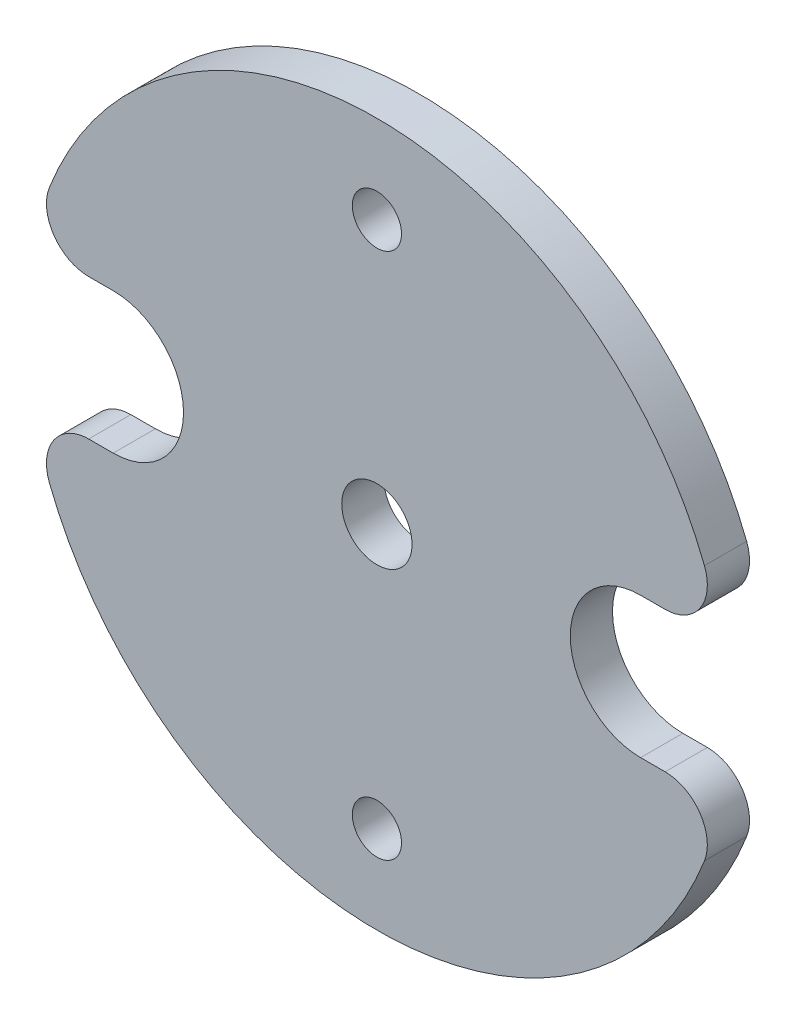
SolidWorks part; units mm, degrees
material "Plain Carbon Steel"
ref_plane "Front Plane" through (0, 0, 0) normal (0, 0, 1) x (1, 0, 0)
ref_plane "Top Plane" through (0, 0, 0) normal (0, 1, 0) x (1, 0, 0)
ref_plane "Right Plane" through (0, 0, 0) normal (1, 0, 0) x (0, 0, -1)
sketch "Plate Profile Sketch" plane through (0, 0, 0) normal (0, 0, 1) x (1, 0, 0)
  line L0 (-19.05, 5.08) -> (-24.8868, 5.08)
  line L1 (-19.05, -5.08) -> (-24.8868, -5.08)
  line L2 (0, 0) -> (0, 16.622) construction
  line L3 (19.05, -5.08) -> (24.8868, -5.08)
  line L4 (19.05, 5.08) -> (24.8868, 5.08)
  arc A0 (-24.8868, -5.08) -> (24.8868, -5.08) centre (0, 0) ccw
  circle A1 centre (0, 0) radius 19.05 construction
  arc A2 (-19.05, -5.08) -> (-19.05, 5.08) centre (-19.05, 0) ccw
  arc A3 (19.05, -5.08) -> (19.05, 5.08) centre (19.05, 0) cw
  arc A4 (24.8868, 5.08) -> (-24.8868, 5.08) centre (0, 0) ccw
  circle A5 centre (0, 19.05) radius 1.778
  circle A6 centre (0, -19.05) radius 1.778
  circle A7 centre (0, 0) radius 2.54
  dimension "D1" = 50.8
  dimension "D2" = 38.1
  dimension "D3" = 10.16
  dimension "D4" = 3.556
  dimension "D5" = 5.08
extrude "Plate Body 0.12in" add sketch "Plate Profile Sketch" along normal blind 3.048
fillet "Fillets R0.12in" radius 3.048 4 edges at (24.8868, -5.08, 1.524) (24.8868, 5.08, 1.524) (-24.8868, 5.08, 1.524) (-24.8868, -5.08, 1.524)
